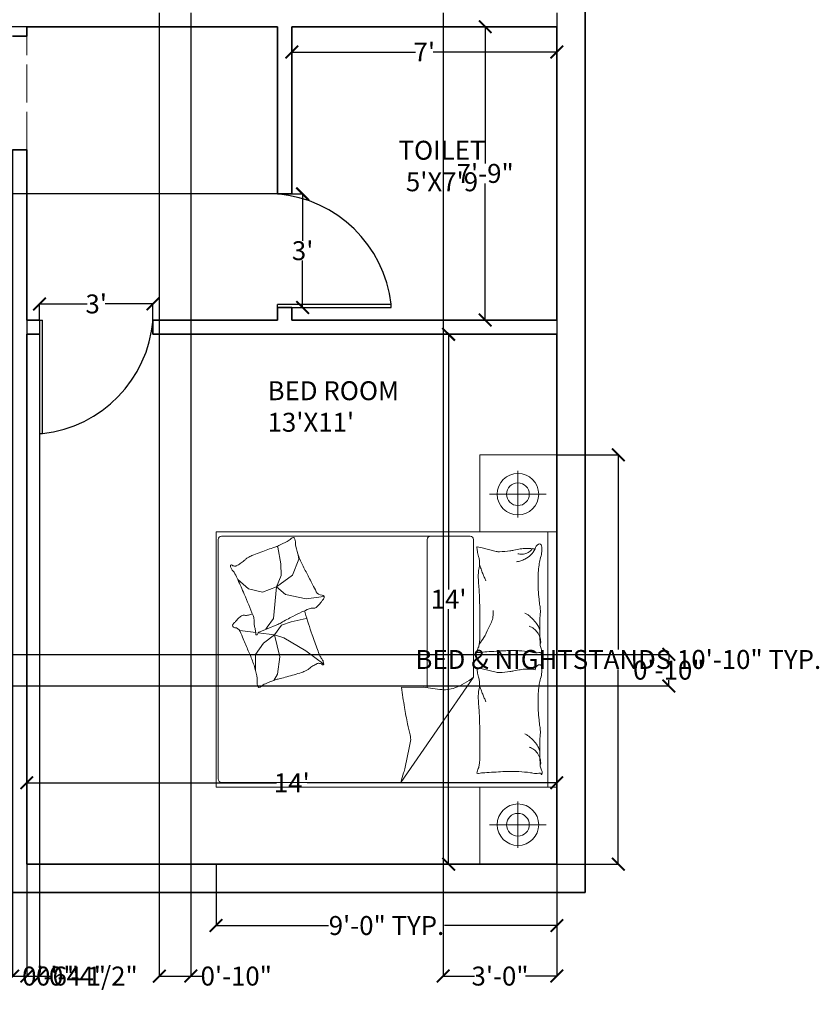
# Model space of a CAD drawing. Units: inches. Extents: x 43 to 543, y 36 to 629.
# Tile 3 of 5: x 290 to 543, y 36 to 348. Entities that reach past the tile are written whole.
import ezdxf

# ---------------------------------------------------------------- set-up
doc = ezdxf.new("R2010")
doc.units = ezdxf.units.IN
doc.header["$MEASUREMENT"] = 0
doc.linetypes.add('ACAD_ISO02W100', pattern=[15, 12, -3])
for name, color, linetype, lineweight in [('A-ANNO-DIMS', 2, 'Continuous', 18), ('A-AREA-IDEN', 7, 'Continuous', 25), ('A-DOOR', 3, 'Continuous', 25), ('A-FURN', 8, 'Continuous', 13), ('A-WALL', 7, 'Continuous', 35), ('A-WALL-OVHD', 7, 'ACAD_ISO02W100', 18)]:
    doc.layers.add(name, color=color, linetype=linetype, lineweight=lineweight)
doc.styles.add('DIM_FONT', font='SIMPLEX.shx', dxfattribs={"width": 0.8})
doc.styles.get("Standard").update_dxf_attribs({"font": 'arial.ttf'})
doc.dimstyles.get("Standard").update_dxf_attribs({"dimtxt": 6, "dimasz": 4, "dimexe": 0.18, "dimexo": 0.0625, "dimgap": 0.09, "dimtad": 0, "dimtih": 1, "dimtoh": 1, "dimdec": 0, "dimzin": 0, "dimdsep": 46, "dimlunit": 4, "dimtxsty": 'Standard', "dimblk": 'ARCHTICK', "dimcen": 0.09, "dimadec": 0, "dimazin": 0, "dimtfac": 1, "dimtdec": 0, "dimtofl": 0, "dimtmove": 0, "dimatfit": 3, "dimldrblk": 'ARCHTICK', "dimfxl": 1, "dimtolj": 1, "dimtzin": 0, "dimarcsym": 1})

# ---------------------------------------------------------------- blocks, each defined once
blk = doc.blocks.new('XDCGFBHJNK')
for p, q in [((549.02, 46.3), (549.02, 41.8)), ((549.02, 46.3), (549.02, 10.3)), ((549.02, 46.3), (550.02, 46.3)), ((550.02, 10.3), (550.02, 46.3)), ((549.02, 10.3), (550.02, 10.3))]:
    blk.add_line(p, q)
blk.add_arc((545.53, 49.68), 39.64, 276.512, 355.1019)
blk = doc.blocks.new('_ArchTick')
at = {"color": 0, "linetype": 'ByBlock', "const_width": 0.15}
blk.add_lwpolyline([(-0.5, -0.5), (0.5, 0.5)], dxfattribs=at)
blk = doc.blocks.new('*D12')
at = {"layer": 'A-ANNO-DIMS', "color": 0, "lineweight": -2, "transparency": 16777216}
for p, q in [((459.82, 248.02), (425.4, 248.02)), ((425.58, 248.02), (425.58, 167.12)), ((425.58, 80.02), (425.58, 160.91)), ((459.82, 80.02), (425.4, 80.02))]:
    blk.add_line(p, q, dxfattribs=at)
at = {"layer": 'Defpoints', "color": 0, "transparency": 16777216}
for p in [(459.88, 248.02), (425.58, 80.02), (459.88, 80.02)]:
    blk.add_point(p, dxfattribs=at)
at = {"layer": 'A-ANNO-DIMS', "color": 0, "lineweight": -2, "transparency": 16777216, "xscale": 4, "yscale": 4, "zscale": 4}
for p, rotation in [((425.58, 248.02), 90), ((425.58, 80.02), 270)]:
    blk.add_blockref('_ArchTick', p, dxfattribs=dict(at, rotation=rotation))
at = {"layer": 'A-ANNO-DIMS', "color": 0, "transparency": 16777216, "insert": (425.58, 164.02), "char_height": 6, "attachment_point": 5}
blk.add_mtext("\\A1;14'", dxfattribs=at)
blk = doc.blocks.new('*D13')
at = {"layer": 'A-ANNO-DIMS', "color": 0, "lineweight": -2, "transparency": 16777216}
for p, q in [((291.88, 80.08), (291.88, 105.97)), ((291.88, 105.79), (370.98, 105.79)), ((459.88, 105.79), (380.78, 105.79)), ((459.88, 80.08), (459.88, 105.97))]:
    blk.add_line(p, q, dxfattribs=at)
at = {"layer": 'Defpoints', "color": 0, "transparency": 16777216}
for p in [(291.88, 105.79), (291.88, 80.02), (459.88, 80.02)]:
    blk.add_point(p, dxfattribs=at)
at = {"layer": 'A-ANNO-DIMS', "color": 0, "lineweight": -2, "transparency": 16777216, "xscale": 4, "yscale": 4, "zscale": 4, "rotation": 180}
blk.add_blockref('_ArchTick', (291.88, 105.79), dxfattribs=at)
at = {"layer": 'A-ANNO-DIMS', "color": 0, "lineweight": -2, "transparency": 16777216, "xscale": 4, "yscale": 4, "zscale": 4}
blk.add_blockref('_ArchTick', (459.88, 105.79), dxfattribs=at)
at = {"layer": 'A-ANNO-DIMS', "color": 0, "transparency": 16777216, "insert": (375.88, 105.79), "char_height": 6, "attachment_point": 5}
blk.add_mtext("\\A1;14'", dxfattribs=at)
blk = doc.blocks.new('*D14')
at = {"layer": 'A-ANNO-DIMS', "color": 0, "lineweight": -2, "transparency": 16777216}
for p, q in [((459.82, 345.52), (437, 345.52)), ((437.18, 345.52), (437.18, 302.17)), ((437.18, 252.52), (437.18, 295.86)), ((459.82, 252.52), (437, 252.52))]:
    blk.add_line(p, q, dxfattribs=at)
at = {"layer": 'Defpoints', "color": 0, "transparency": 16777216}
for p in [(459.88, 345.52), (437.18, 252.52), (459.88, 252.52)]:
    blk.add_point(p, dxfattribs=at)
at = {"layer": 'A-ANNO-DIMS', "color": 0, "lineweight": -2, "transparency": 16777216, "xscale": 4, "yscale": 4, "zscale": 4}
for p, rotation in [((437.18, 345.52), 90), ((437.18, 252.52), 270)]:
    blk.add_blockref('_ArchTick', p, dxfattribs=dict(at, rotation=rotation))
at = {"layer": 'A-ANNO-DIMS', "color": 0, "transparency": 16777216, "insert": (437.18, 299.02), "char_height": 6, "attachment_point": 5}
blk.add_mtext('\\A1;7\'-9"', dxfattribs=at)
blk = doc.blocks.new('*D15')
at = {"layer": 'A-ANNO-DIMS', "color": 0, "lineweight": -2, "transparency": 16777216}
for p, q in [((375.88, 345.45), (375.88, 337.34)), ((459.88, 345.45), (459.88, 337.34)), ((375.88, 337.52), (415.05, 337.52)), ((459.88, 337.52), (420.7, 337.52))]:
    blk.add_line(p, q, dxfattribs=at)
at = {"layer": 'Defpoints', "color": 0, "transparency": 16777216}
for p in [(375.88, 345.52), (459.88, 345.52), (459.88, 337.52)]:
    blk.add_point(p, dxfattribs=at)
at = {"layer": 'A-ANNO-DIMS', "color": 0, "lineweight": -2, "transparency": 16777216, "xscale": 4, "yscale": 4, "zscale": 4, "rotation": 180}
blk.add_blockref('_ArchTick', (375.88, 337.52), dxfattribs=at)
at = {"layer": 'A-ANNO-DIMS', "color": 0, "lineweight": -2, "transparency": 16777216, "xscale": 4, "yscale": 4, "zscale": 4}
blk.add_blockref('_ArchTick', (459.88, 337.52), dxfattribs=at)
at = {"layer": 'A-ANNO-DIMS', "color": 0, "transparency": 16777216, "insert": (417.88, 337.52), "char_height": 6, "attachment_point": 5}
blk.add_mtext("\\A1;7'", dxfattribs=at)
blk = doc.blocks.new('*D20')
at = {"layer": 'A-ANNO-DIMS', "color": 0, "lineweight": -2, "transparency": 16777216}
for p, q in [((295.88, 252.58), (295.88, 257.82)), ((295.88, 257.64), (311.03, 257.64)), ((331.88, 257.64), (316.73, 257.64)), ((331.88, 252.58), (331.88, 257.82))]:
    blk.add_line(p, q, dxfattribs=at)
at = {"layer": 'Defpoints', "color": 0, "transparency": 16777216}
for p in [(295.88, 257.64), (295.88, 252.52), (331.88, 252.52)]:
    blk.add_point(p, dxfattribs=at)
at = {"layer": 'A-ANNO-DIMS', "color": 0, "lineweight": -2, "transparency": 16777216, "xscale": 4, "yscale": 4, "zscale": 4, "rotation": 180}
blk.add_blockref('_ArchTick', (295.88, 257.64), dxfattribs=at)
at = {"layer": 'A-ANNO-DIMS', "color": 0, "lineweight": -2, "transparency": 16777216, "xscale": 4, "yscale": 4, "zscale": 4}
blk.add_blockref('_ArchTick', (331.88, 257.64), dxfattribs=at)
at = {"layer": 'A-ANNO-DIMS', "color": 0, "transparency": 16777216, "insert": (313.88, 257.64), "char_height": 6, "attachment_point": 5}
blk.add_mtext("\\A1;3'", dxfattribs=at)
blk = doc.blocks.new('*D21')
at = {"layer": 'A-ANNO-DIMS', "color": 0, "lineweight": -2, "transparency": 16777216}
for p, q in [((371.44, 292.52), (379.48, 292.52)), ((379.3, 292.52), (379.3, 277.67)), ((379.3, 256.52), (379.3, 271.36)), ((371.44, 256.52), (379.48, 256.52))]:
    blk.add_line(p, q, dxfattribs=at)
at = {"layer": 'Defpoints', "color": 0, "transparency": 16777216}
for p in [(371.38, 292.52), (371.38, 256.52), (379.3, 256.52)]:
    blk.add_point(p, dxfattribs=at)
at = {"layer": 'A-ANNO-DIMS', "color": 0, "lineweight": -2, "transparency": 16777216, "xscale": 4, "yscale": 4, "zscale": 4}
for p, rotation in [((379.3, 292.52), 90), ((379.3, 256.52), 270)]:
    blk.add_blockref('_ArchTick', p, dxfattribs=dict(at, rotation=rotation))
at = {"layer": 'A-ANNO-DIMS', "color": 0, "transparency": 16777216, "insert": (379.3, 274.52), "char_height": 6, "attachment_point": 5}
blk.add_mtext("\\A1;3'", dxfattribs=at)
blk = doc.blocks.new('BED-DOUBLE-WITH-NIGHTSTANDS')
for p, q in [((83.62, 105.4), (83.62, 129.79)), ((83.62, 129.79), (108, 129.79)), ((108, 129.79), (108, 105.4)), ((95.68, 109.93), (95.68, 124.65)), ((104.67, 117.29), (86.69, 117.29)), ((80.54, 104), (1.74, 104)), ((105.17, 105.4), (105.17, 24.4)), ((0.66, 102.92), (0.66, 27.01)), ((19.54, 100.52), (19.19, 100.7)), ((20.47, 95.22), (19.54, 100.52)), ((66.9, 102.92), (66.9, 55.97)), ((81.62, 59.31), (81.62, 102.92)), ((26.22, 96.71), (26.04, 98.01)), ((20.65, 91.51), (20.47, 95.22)), ((24.18, 91.6), (26.22, 96.71)), ((19.17, 87.89), (24.18, 91.6)), ((19.17, 87.89), (20.65, 91.51)), ((10.26, 87.33), (6.88, 90.22)), ((19.17, 87.89), (14.71, 86.21)), ((19.17, 87.89), (18.15, 77.85)), ((21.95, 85.47), (19.17, 87.89)), ((14.71, 86.21), (10.26, 87.33)), ((28.54, 84.08), (21.95, 85.47)), ((34.11, 84.82), (28.54, 84.08)), ((16.2, 75.16), (15.73, 74.51)), ((18.15, 77.85), (16.2, 75.16)), ((18.47, 72.7), (20.71, 75.8)), ((20.71, 75.8), (23.8, 76.86)), ((23.8, 76.86), (28.6, 77.93)), ((12.59, 73.43), (7.48, 74.07)), ((18.47, 72.7), (13.38, 73.34)), ((18.47, 72.7), (15.05, 70.03)), ((21.45, 71.74), (18.47, 72.7)), ((18.47, 72.7), (20.17, 65.76)), ((15.05, 70.03), (12.49, 66.51)), ((28.49, 67.68), (21.45, 71.74)), ((12.49, 66.51), (12.49, 61.49)), ((20.17, 65.76), (19.43, 60.21)), ((34.11, 63.41), (28.49, 67.68)), ((19.43, 60.21), (18.34, 58.27)), ((81.62, 59.31), (58.54, 25.93)), ((1.74, 25.93), (58.54, 25.93)), ((83.62, 24.4), (83.62, 0)), ((108, 0), (108, 24.4)), ((95.68, 19.86), (95.68, 5.14)), ((104.67, 12.5), (86.69, 12.5)), ((83.62, 0), (108, 0))]:
    blk.add_line(p, q)
blk.add_lwpolyline([(0, 105.4), (108, 105.4), (108, 24.4), (0, 24.4)], close=True)
blk.add_lwpolyline([(22.51, 102.26, 0.101392), (23.8, 103.26, -0.223768), (24.5, 103.58, -0.25558), (24.77, 103.43, -0.081563), (25.1, 102.61, -0.071805), (25.18, 101.69, 0.069985), (25.26, 100.74, 0.03546), (26.2, 97.59, 0.029432), (27.82, 93.98, 0.001554), (28.73, 92.24, -0.00152), (29.66, 90.47, -0.004735), (30.6, 88.63, 0.00382), (31.75, 86.35, 0.296001), (33.58, 85.3, -0.649774), (34.16, 84.19, -0.02319), (33.93, 83.92, 0.0288), (33.74, 83.71, 0.005727), (33.46, 83.33, -0.004358), (33.09, 82.83, -0.027528), (32.25, 81.85, -0.046214), (31.67, 81.34, -0.194121), (30.78, 81.12, 0.133719), (29.49, 80.96, 0.011505), (27.21, 79.95, 0.008882), (24.3, 78.53, 0.012426), (20.61, 76.53, -0.033612), (19.21, 75.84), (16.17, 74.6), (13.82, 73.64, 0.224341), (13.11, 72.86, -0.722772), (12.63, 72.85, -0.103513), (12.6, 73.05, 0.053465), (12.59, 73.44, 0.030109), (12.34, 74.68, -0.031436), (12.1, 75.88, -0.05324), (12.08, 76.69, 0.05518), (12.05, 77.48, 0.056271), (11.7, 78.85, 0.0108), (8.92, 85.64, 0.00456), (6.88, 90.22, 0.01125), (5.99, 92.05, 0.069394), (5.31, 93.02, -0.079756), (4.74, 93.88, -0.106399), (4.57, 94.66, -0.328642), (4.73, 94.89, -0.299547), (5.09, 94.79, 0.189917), (5.59, 94.53, 0.033518), (6.15, 94.51, 0.075627), (6.39, 94.55, 0.053489), (6.8, 94.74, 0.017838), (7.94, 95.49, 0.038394), (9.17, 96.51, -0.059529), (10, 97.14, -0.035943), (11.36, 97.82, -0.011245), (15.91, 99.56, -0.006203), (17.99, 100.27, 0.010783), (19.19, 100.7, 0.019485), (19.89, 100.99, 0.005062)], format="xyb", close=True)
for points in [[(101.15, 99.94, -0.263368), (102.17, 101.45, -0.494818), (103.18, 100.96, -0.049225), (103.27, 100, -0.036831), (103.18, 98.73, -0.031893), (102.74, 96.68, 0.035782), (102.36, 94.84, 0.032941), (102.04, 90, 0.026564), (102.36, 84, 0.017905), (102.65, 81.97, -0.033397), (102.77, 80.88, -0.03204), (102.73, 78.88, 0.018442), (102.57, 75.4, 0.010837), (102.61, 71.91, 0.014624), (102.77, 69.32, 0.111249), (103.17, 68.1, -0.153708), (103.38, 67.19, -0.076444), (103.29, 66.79, -0.215512), (103.18, 66.68, -0.585858), (103.02, 66.83, 0.363489), (102.88, 67.09, 0.191716), (102.25, 67.09, -0.129675), (101.36, 66.99, -0.01735), (100.45, 67.15, 0.019326), (99.63, 67.29, 0.018818), (95.94, 67.65, 0.021828), (92.74, 67.7, 0.006204), (90.91, 67.62, 0.001963), (85.14, 67.29, 0.028341), (83.19, 67.06, -0.117014), (82.71, 67.09, -0.36606), (82.66, 67.17, -0.03973), (82.81, 67.9, -0.048309), (83.11, 68.64, 0.062981), (83.32, 69.22, 0.04058), (83.5, 70.48, 0.014345), (83.62, 74.08, 0.005484), (83.58, 80.86, 0.007153), (83.42, 86.05, 0.008762), (83.27, 88.35, -0.008153), (83.12, 90.82, -0.06251), (83.35, 93.9, 0.078669), (83.46, 96.36, 0.047825), (83.21, 97.57, -0.034494), (82.81, 99.23, -0.023571), (82.65, 100.6, -0.510228), (82.71, 100.65), (84.33, 100.25), (88.79, 99.13, 0.073041), (89.85, 99.03, 0.023305), (93.15, 99.33, 0.018299), (94.38, 99.55, -0.01097), (96.43, 99.95, -0.042281), (98.29, 100.11, -0.027201), (101.17, 99.95)], [(101.15, 99.95, -0.077379), (99.79, 98.07, -0.077379), (97.91, 96.7, -0.047525), (96.58, 96.16, -0.047525), (95.17, 95.89)], [(100.29, 100.03, -0.05369), (99.59, 99.27, -0.070312), (98.92, 98.83, -0.015448), (98.46, 98.63, -0.013244), (97.91, 98.42, -0.082127), (96.93, 98.26, -0.064164), (95.68, 98.42)], [(83.5, 95.06, 0.009729), (83.99, 93.59, 0.009729), (84.53, 92.13, 0.007971), (85.02, 90.96, 0.007971), (85.55, 89.8)], [(28.06, 80.34, 0.025626), (28.21, 79.72, 0.0108), (30.46, 72.73, 0.00456), (32.14, 68.01, 0.01125), (32.88, 66.11, 0.069394), (33.49, 65.1, -0.079756), (33.99, 64.2, -0.106399), (34.11, 63.41, -0.328642), (33.92, 63.19, -0.299547), (33.57, 63.32, 0.189917), (33.1, 63.62, 0.033518), (32.54, 63.68, 0.075627), (32.29, 63.65, 0.053489), (31.87, 63.49, 0.017838), (30.68, 62.84, 0.038394), (29.37, 61.91, -0.059529), (28.5, 61.35, -0.035943), (27.09, 60.78, -0.011245), (22.42, 59.39, -0.006203), (20.29, 58.84, 0.010783), (19.06, 58.51, 0.019485), (18.34, 58.27, 0.005062), (15.63, 57.21, 0.101392), (14.27, 56.3, -0.223768), (13.54, 56.04, -0.25558), (13.29, 56.21, -0.081563), (13.02, 57.06, -0.071805), (13.01, 57.98, 0.069985), (13.01, 58.93, 0.03546), (12.31, 62.14, 0.029432), (10.97, 65.87, 0.001554), (10.2, 67.67, -0.00152), (9.41, 69.51, -0.004735), (8.61, 71.41, 0.00382), (7.64, 73.78, 0.296001), (5.89, 74.96, -0.649774), (5.41, 76.12, -0.02319), (5.66, 76.36, 0.0288), (5.85, 76.56, 0.005727), (6.17, 76.91, -0.004358), (6.58, 77.38, -0.027528), (7.49, 78.3, -0.046214), (8.1, 78.76, -0.194121), (9, 78.91, 0.133719), (10.3, 78.98, 0.005779), (11.49, 79.38, 0.008882)], [(83.42, 69.72, 0.016108), (84.84, 71.83, 0.024599), (85.65, 73.27, 0.009477), (86.91, 75.92, 0.015937), (87.57, 77.53, 0.072521), (87.77, 78.41, 0.033339), (87.78, 80.37)], [(102.57, 74.35, 0.027842), (101.99, 75.64, 0.048685), (101.56, 76.32, 0.023666), (100.24, 77.82, 0.031223), (99.13, 78.85, 0.046801), (98.71, 79.13, 0.023191), (97.81, 79.56)], [(102.88, 69.93, 0.088153), (102.68, 71.79, 0.088153), (101.86, 73.48, 0.077547), (100.7, 74.65, 0.077547), (99.23, 75.4)], [(101.15, 61.64, -0.263368), (102.17, 63.15, -0.494818), (103.18, 62.66, -0.049225), (103.27, 61.7, -0.036831), (103.18, 60.43, -0.031893), (102.74, 58.38, 0.035782), (102.36, 56.55, 0.032941), (102.04, 51.7, 0.026564), (102.36, 45.7, 0.017905), (102.65, 43.67, -0.033397), (102.77, 42.58, -0.03204), (102.73, 40.58, 0.018442), (102.57, 37.1, 0.010837), (102.61, 33.61, 0.014624), (102.77, 31.02, 0.111249), (103.17, 29.8, -0.153708), (103.38, 28.89, -0.076444), (103.29, 28.49, -0.215512), (103.18, 28.38, -0.585858), (103.02, 28.53, 0.363489), (102.88, 28.79, 0.191716), (102.25, 28.79, -0.129675), (101.36, 28.69, -0.01735), (100.45, 28.85, 0.019326), (99.63, 28.99, 0.018818), (95.94, 29.35, 0.021828), (92.74, 29.4, 0.006204), (90.91, 29.32, 0.001963), (85.14, 28.99, 0.028341), (83.19, 28.76, -0.117014), (82.71, 28.79, -0.36606), (82.66, 28.87, -0.03973), (82.81, 29.6, -0.048309), (83.11, 30.34, 0.062981), (83.32, 30.92, 0.04058), (83.5, 32.18, 0.014345), (83.62, 35.79, 0.005484), (83.58, 42.56, 0.007153), (83.42, 47.75, 0.008762), (83.27, 50.05, -0.008153), (83.12, 52.52, -0.06251), (83.35, 55.6, 0.078669), (83.46, 58.06, 0.047825), (83.21, 59.27, -0.034494), (82.81, 60.93, -0.023571), (82.65, 62.3, -0.510228), (82.71, 62.35), (84.33, 61.95), (88.79, 60.83, 0.073041), (89.85, 60.73, 0.023305), (93.15, 61.04, 0.018299), (94.38, 61.26, -0.01097), (96.43, 61.65, -0.042281), (98.29, 61.81, -0.027201), (101.17, 61.65)], [(81.62, 59.31, -0.085272), (75.67, 55.89, -0.124044), (70.95, 55.39), (65.79, 56.13), (58.77, 56.03)], [(83.5, 56.76, 0.009729), (83.99, 55.29, 0.009729), (84.53, 53.84, 0.007971), (85.02, 52.66, 0.007971), (85.55, 51.5)], [(58.77, 56.03, 0.007867), (59.73, 49.68, 0.009508), (60.7, 44.46, 0.006616), (61.48, 40.95, -0.023828), (61.66, 39.97, -0.080713), (61.63, 38.96, -0.009591), (59.91, 30.72, -0.013133), (59.44, 28.91, -0.007859), (58.54, 25.93)], [(102.57, 36.06, 0.027842), (101.99, 37.34, 0.048685), (101.56, 38.02, 0.023666), (100.24, 39.52, 0.031223), (99.13, 40.55, 0.046801), (98.71, 40.83, 0.023191), (97.81, 41.26)], [(102.88, 31.63, 0.088153), (102.68, 33.49, 0.088153), (101.86, 35.18, 0.077547), (100.7, 36.35, 0.077547), (99.23, 37.1)]]:
    blk.add_lwpolyline(points, format="xyb")
for centre, radius in [((95.68, 117.29), 6.58), ((95.68, 117.29), 3.6), ((95.68, 12.5), 6.58), ((95.68, 12.5), 3.6)]:
    blk.add_circle(centre, radius)
for centre, start, end in [((1.74, 102.92), 90, 180), ((67.98, 102.92), 90, 180), ((80.54, 102.92), 0, 90), ((1.74, 27.01), 180, 270)]:
    blk.add_arc(centre, 1.08, start, end)
at = {"style": 'DIM_FONT', "width": 0.8, "flags": 9}
for tag in ['YSIZE', 'XSIZE']:
    blk.add_attdef(tag, (108, 105.4), '', height=0.027, rotation=270, dxfattribs=at)
blk = doc.blocks.new('*D27')
at = {"layer": 'A-ANNO-DIMS', "color": 0, "lineweight": -2, "transparency": 16777216}
for p, q in [((459.97, 209.81), (479.55, 209.81)), ((479.37, 209.81), (479.37, 148.12)), ((479.37, 80.02), (479.37, 141.7)), ((459.97, 80.02), (479.55, 80.02))]:
    blk.add_line(p, q, dxfattribs=at)
at = {"layer": 'Defpoints', "color": 0, "transparency": 16777216}
for p in [(459.9, 209.81), (479.37, 209.81), (459.9, 80.02)]:
    blk.add_point(p, dxfattribs=at)
at = {"layer": 'A-ANNO-DIMS', "color": 0, "lineweight": -2, "transparency": 16777216, "xscale": 4, "yscale": 4, "zscale": 4}
for p, rotation in [((479.37, 209.81), 90), ((479.37, 80.02), 270)]:
    blk.add_blockref('_ArchTick', p, dxfattribs=dict(at, rotation=rotation))
at = {"layer": 'A-ANNO-DIMS', "color": 0, "transparency": 16777216, "insert": (479.37, 144.91), "char_height": 6, "attachment_point": 5}
blk.add_mtext('\\A1;BED & NIGHTSTANDS 10\'-10" TYP.', dxfattribs=at)
blk = doc.blocks.new('*D28')
at = {"layer": 'A-ANNO-DIMS', "color": 0, "lineweight": -2, "transparency": 16777216}
for p, q in [((351.88, 79.95), (351.88, 60.37)), ((459.9, 79.95), (459.9, 60.37)), ((351.88, 60.55), (387.51, 60.55)), ((459.9, 60.55), (424.27, 60.55))]:
    blk.add_line(p, q, dxfattribs=at)
at = {"layer": 'Defpoints', "color": 0, "transparency": 16777216}
for p in [(351.88, 80.02), (459.9, 80.02), (459.9, 60.55)]:
    blk.add_point(p, dxfattribs=at)
at = {"layer": 'A-ANNO-DIMS', "color": 0, "lineweight": -2, "transparency": 16777216, "xscale": 4, "yscale": 4, "zscale": 4, "rotation": 180}
blk.add_blockref('_ArchTick', (351.88, 60.55), dxfattribs=at)
at = {"layer": 'A-ANNO-DIMS', "color": 0, "lineweight": -2, "transparency": 16777216, "xscale": 4, "yscale": 4, "zscale": 4}
blk.add_blockref('_ArchTick', (459.9, 60.55), dxfattribs=at)
at = {"layer": 'A-ANNO-DIMS', "color": 0, "transparency": 16777216, "insert": (405.89, 60.55), "char_height": 6, "attachment_point": 5}
blk.add_mtext('\\A1;9\'-0" TYP.', dxfattribs=at)
blk = doc.blocks.new('*D36')
at = {"layer": 'A-ANNO-DIMS', "color": 0, "lineweight": -2, "transparency": 16777216}
for p, q in [((459.88, 363.72), (459.88, 356.4)), ((468.88, 363.72), (468.88, 356.4)), ((459.88, 356.58), (468.88, 356.58)), ((468.88, 356.58), (472.88, 356.58))]:
    blk.add_line(p, q, dxfattribs=at)
at = {"layer": 'Defpoints', "color": 0, "transparency": 16777216}
for p in [(459.88, 363.78), (468.88, 363.78), (468.88, 356.58)]:
    blk.add_point(p, dxfattribs=at)
at = {"layer": 'A-ANNO-DIMS', "color": 0, "lineweight": -2, "transparency": 16777216, "xscale": 4, "yscale": 4, "zscale": 4, "rotation": 180}
blk.add_blockref('_ArchTick', (459.88, 356.58), dxfattribs=at)
at = {"layer": 'A-ANNO-DIMS', "color": 0, "lineweight": -2, "transparency": 16777216, "xscale": 4, "yscale": 4, "zscale": 4}
blk.add_blockref('_ArchTick', (468.88, 356.58), dxfattribs=at)
at = {"layer": 'A-ANNO-DIMS', "color": 0, "transparency": 16777216, "insert": (491.25, 356.58), "char_height": 6, "attachment_point": 5}
blk.add_mtext('\\A1;0\'-9" TYP.', dxfattribs=at)
blk = doc.blocks.new('*D42')
at = {"layer": 'A-ANNO-DIMS', "color": 0, "lineweight": -2, "transparency": 16777216}
for p, q in [((281.38, 156.45), (281.38, 44.34)), ((287.38, 156.45), (287.38, 44.34)), ((281.38, 44.52), (287.38, 44.52)), ((287.38, 44.52), (291.38, 44.52))]:
    blk.add_line(p, q, dxfattribs=at)
at = {"layer": 'Defpoints', "color": 0, "transparency": 16777216}
for p in [(281.38, 156.52), (287.38, 156.52), (287.38, 44.52)]:
    blk.add_point(p, dxfattribs=at)
at = {"layer": 'A-ANNO-DIMS', "color": 0, "lineweight": -2, "transparency": 16777216, "xscale": 4, "yscale": 4, "zscale": 4, "rotation": 180}
blk.add_blockref('_ArchTick', (281.38, 44.52), dxfattribs=at)
at = {"layer": 'A-ANNO-DIMS', "color": 0, "lineweight": -2, "transparency": 16777216, "xscale": 4, "yscale": 4, "zscale": 4}
blk.add_blockref('_ArchTick', (287.38, 44.52), dxfattribs=at)
at = {"layer": 'A-ANNO-DIMS', "color": 0, "transparency": 16777216, "insert": (299.44, 44.52), "char_height": 6, "attachment_point": 5}
blk.add_mtext('\\A1;0\'-6"', dxfattribs=at)
blk = doc.blocks.new('*D47')
at = {"layer": 'A-ANNO-DIMS', "color": 0, "lineweight": -2, "transparency": 16777216}
for p, q in [((423.88, 349.95), (423.88, 44.34)), ((459.88, 349.95), (459.88, 44.34)), ((423.88, 44.52), (433.81, 44.52)), ((459.88, 44.52), (449.94, 44.52))]:
    blk.add_line(p, q, dxfattribs=at)
at = {"layer": 'Defpoints', "color": 0, "transparency": 16777216}
for p in [(423.88, 350.02), (459.88, 350.02), (459.88, 44.52)]:
    blk.add_point(p, dxfattribs=at)
at = {"layer": 'A-ANNO-DIMS', "color": 0, "lineweight": -2, "transparency": 16777216, "xscale": 4, "yscale": 4, "zscale": 4, "rotation": 180}
blk.add_blockref('_ArchTick', (423.88, 44.52), dxfattribs=at)
at = {"layer": 'A-ANNO-DIMS', "color": 0, "lineweight": -2, "transparency": 16777216, "xscale": 4, "yscale": 4, "zscale": 4}
blk.add_blockref('_ArchTick', (459.88, 44.52), dxfattribs=at)
at = {"layer": 'A-ANNO-DIMS', "color": 0, "transparency": 16777216, "insert": (441.88, 44.52), "char_height": 6, "attachment_point": 5}
blk.add_mtext('\\A1;3\'-0"', dxfattribs=at)
blk = doc.blocks.new('*D48')
at = {"layer": 'A-ANNO-DIMS', "color": 0, "lineweight": -2, "transparency": 16777216}
for p, q in [((333.88, 349.95), (333.88, 44.34)), ((343.88, 349.95), (343.88, 44.34)), ((333.88, 44.52), (343.88, 44.52)), ((343.88, 44.52), (347.88, 44.52))]:
    blk.add_line(p, q, dxfattribs=at)
at = {"layer": 'Defpoints', "color": 0, "transparency": 16777216}
for p in [(333.88, 350.02), (343.88, 350.02), (343.88, 44.52)]:
    blk.add_point(p, dxfattribs=at)
at = {"layer": 'A-ANNO-DIMS', "color": 0, "lineweight": -2, "transparency": 16777216, "xscale": 4, "yscale": 4, "zscale": 4, "rotation": 180}
blk.add_blockref('_ArchTick', (333.88, 44.52), dxfattribs=at)
at = {"layer": 'A-ANNO-DIMS', "color": 0, "lineweight": -2, "transparency": 16777216, "xscale": 4, "yscale": 4, "zscale": 4}
blk.add_blockref('_ArchTick', (343.88, 44.52), dxfattribs=at)
at = {"layer": 'A-ANNO-DIMS', "color": 0, "transparency": 16777216, "insert": (358.27, 44.52), "char_height": 6, "attachment_point": 5}
blk.add_mtext('\\A1;0\'-10"', dxfattribs=at)
blk = doc.blocks.new('*D49')
at = {"layer": 'A-ANNO-DIMS', "color": 0, "lineweight": -2, "transparency": 16777216}
for p, q in [((371.32, 345.52), (58.2, 345.52)), ((58.38, 345.52), (58.38, 322.16)), ((58.38, 292.52), (58.38, 315.88)), ((371.32, 292.52), (58.2, 292.52))]:
    blk.add_line(p, q, dxfattribs=at)
at = {"layer": 'Defpoints', "color": 0, "transparency": 16777216}
for p in [(58.38, 345.52), (371.38, 345.52), (371.38, 292.52)]:
    blk.add_point(p, dxfattribs=at)
at = {"layer": 'A-ANNO-DIMS', "color": 0, "lineweight": -2, "transparency": 16777216, "xscale": 4, "yscale": 4, "zscale": 4}
for p, rotation in [((58.38, 345.52), 90), ((58.38, 292.52), 270)]:
    blk.add_blockref('_ArchTick', p, dxfattribs=dict(at, rotation=rotation))
at = {"layer": 'A-ANNO-DIMS', "color": 0, "transparency": 16777216, "insert": (58.38, 319.02), "char_height": 6, "attachment_point": 5}
blk.add_mtext('\\A1;4\'-5"', dxfattribs=at)
blk = doc.blocks.new('*D62')
at = {"layer": 'A-ANNO-DIMS', "color": 0, "lineweight": -2, "transparency": 16777216}
for p, q in [((291.88, 252.45), (291.88, 44.34)), ((295.88, 252.45), (295.88, 44.34)), ((291.88, 44.52), (295.88, 44.52)), ((295.88, 44.52), (299.88, 44.52))]:
    blk.add_line(p, q, dxfattribs=at)
at = {"layer": 'Defpoints', "color": 0, "transparency": 16777216}
for p in [(291.88, 252.52), (295.88, 252.52), (295.88, 44.52)]:
    blk.add_point(p, dxfattribs=at)
at = {"layer": 'A-ANNO-DIMS', "color": 0, "lineweight": -2, "transparency": 16777216, "xscale": 4, "yscale": 4, "zscale": 4, "rotation": 180}
blk.add_blockref('_ArchTick', (291.88, 44.52), dxfattribs=at)
at = {"layer": 'A-ANNO-DIMS', "color": 0, "lineweight": -2, "transparency": 16777216, "xscale": 4, "yscale": 4, "zscale": 4}
blk.add_blockref('_ArchTick', (295.88, 44.52), dxfattribs=at)
at = {"layer": 'A-ANNO-DIMS', "color": 0, "transparency": 16777216, "insert": (307.94, 44.52), "char_height": 6, "attachment_point": 5}
blk.add_mtext('\\A1;0\'-4"', dxfattribs=at)
blk = doc.blocks.new('*D66')
at = {"layer": 'A-ANNO-DIMS', "color": 0, "lineweight": -2, "transparency": 16777216}
for p, q in [((287.44, 146.52), (495.56, 146.52)), ((495.38, 146.52), (495.38, 144.67)), ((495.38, 136.52), (495.38, 138.36)), ((287.44, 136.52), (495.56, 136.52))]:
    blk.add_line(p, q, dxfattribs=at)
at = {"layer": 'Defpoints', "color": 0, "transparency": 16777216}
for p in [(287.38, 146.52), (495.38, 146.52), (287.38, 136.52)]:
    blk.add_point(p, dxfattribs=at)
at = {"layer": 'A-ANNO-DIMS', "color": 0, "lineweight": -2, "transparency": 16777216, "xscale": 4, "yscale": 4, "zscale": 4}
for p, rotation in [((495.38, 146.52), 90), ((495.38, 136.52), 270)]:
    blk.add_blockref('_ArchTick', p, dxfattribs=dict(at, rotation=rotation))
at = {"layer": 'A-ANNO-DIMS', "color": 0, "transparency": 16777216, "insert": (495.38, 141.52), "char_height": 6, "attachment_point": 5}
blk.add_mtext('\\A1;0\'-10"', dxfattribs=at)
blk = doc.blocks.new('*D67')
at = {"layer": 'A-ANNO-DIMS', "color": 0, "lineweight": -2, "transparency": 16777216}
for p, q in [((287.38, 306.45), (287.38, 44.34)), ((291.88, 306.45), (291.88, 44.34)), ((287.38, 44.52), (291.88, 44.52)), ((291.88, 44.52), (295.88, 44.52))]:
    blk.add_line(p, q, dxfattribs=at)
at = {"layer": 'Defpoints', "color": 0, "transparency": 16777216}
for p in [(287.38, 306.52), (291.88, 306.52), (291.88, 44.52)]:
    blk.add_point(p, dxfattribs=at)
at = {"layer": 'A-ANNO-DIMS', "color": 0, "lineweight": -2, "transparency": 16777216, "xscale": 4, "yscale": 4, "zscale": 4, "rotation": 180}
blk.add_blockref('_ArchTick', (287.38, 44.52), dxfattribs=at)
at = {"layer": 'A-ANNO-DIMS', "color": 0, "lineweight": -2, "transparency": 16777216, "xscale": 4, "yscale": 4, "zscale": 4}
blk.add_blockref('_ArchTick', (291.88, 44.52), dxfattribs=at)
at = {"layer": 'A-ANNO-DIMS', "color": 0, "transparency": 16777216, "insert": (310.93, 44.52), "char_height": 6, "attachment_point": 5}
blk.add_mtext('\\A1;0\'-4 1/2"', dxfattribs=at)

msp = doc.modelspace()

# ---------------------------------------------------------------- linework, layer by layer
at = {"layer": 'A-WALL'}
for p, q in [((468.88, 599.02), (468.88, 71.02)), ((291.88, 345.52), (291.88, 342.52)), ((291.88, 345.52), (371.38, 345.52)), ((371.38, 345.52), (371.38, 306.52)), ((375.88, 345.52), (375.88, 306.52)), ((375.88, 345.52), (459.88, 345.52)), ((459.88, 345.52), (459.88, 252.52)), ((287.38, 342.52), (291.88, 342.52)), ((287.38, 306.52), (291.88, 306.52)), ((291.88, 306.52), (291.88, 252.52)), ((371.38, 306.52), (371.38, 292.52)), ((375.88, 306.52), (375.88, 292.52)), ((375.88, 292.52), (371.38, 292.52)), ((375.88, 256.52), (371.38, 256.52)), ((371.38, 256.52), (371.38, 252.52)), ((375.88, 256.52), (375.88, 252.52)), ((295.88, 252.52), (291.88, 252.52)), ((371.38, 252.52), (331.88, 252.52)), ((331.88, 252.52), (331.88, 248.02)), ((459.88, 252.52), (375.88, 252.52)), ((291.88, 248.02), (291.88, 80.02)), ((295.88, 248.02), (291.88, 248.02)), ((459.88, 248.02), (331.88, 248.02)), ((459.88, 248.02), (459.88, 80.02)), ((459.88, 80.02), (291.88, 80.02)), ((468.88, 71.02), (84.88, 71.02))]:
    msp.add_line(p, q, dxfattribs=at)
at = {"layer": 'A-WALL-OVHD'}
for p, q in [((291.88, 342.52), (287.38, 342.52)), ((291.88, 306.52), (291.88, 342.52))]:
    msp.add_line(p, q, dxfattribs=at)

# ---------------------------------------------------------------- block references
at = {"layer": 'A-DOOR', "rotation": 90}
msp.add_blockref('XDCGFBHJNK', (417.67, -292.51), dxfattribs=at)
at = {"layer": 'A-DOOR'}
msp.add_blockref('XDCGFBHJNK', (-253.14, 206.22), dxfattribs=at)
at = {"layer": 'A-FURN'}
msp.add_blockref('BED-DOUBLE-WITH-NIGHTSTANDS', (351.88, 80.02), dxfattribs=at)

# ---------------------------------------------------------------- texts
at = {"layer": 'A-AREA-IDEN', "char_height": 6, "attachment_point": 1}
for s, width, insert in [("\\pxqc;TOILET\\P5'X7'9", 52.429, (397.26, 309.37)), ("BED ROOM\\P13'X11' ", 90.4757, (368.21, 233.12))]:
    msp.add_mtext_dynamic_manual_height_columns(s, width=width, gutter_width=30, heights=[0], dxfattribs=dict(at, insert=insert))

# ---------------------------------------------------------------- dimensions: what is measured, and where the dimension line sits
at = {"layer": 'A-ANNO-DIMS'}
for base, p1, p2, picture, middle in [((468.88, 356.58), (459.88, 363.78), (468.88, 363.78), '*D36', (491.25, 356.58)), ((459.9, 60.55), (351.88, 80.02), (459.9, 80.02), '*D28', (405.89, 60.55))]:
    dim = msp.add_linear_dim(base=base, p1=p1, p2=p2, text='<> TYP.', dimstyle='Standard', override={"dimdec": 1, "dimlfac": 1, "dimrnd": 0, "dimzin": 1, "dimdsep": 46, "dimlunit": 4, "dimfrac": 2}, dxfattribs=at)
    dim.commit()
    dim.dimension.update_dxf_attribs({"geometry": picture, "text_midpoint": middle})
for base, p1, p2, override, picture, middle in [((343.88, 44.52), (333.88, 350.02), (343.88, 350.02), {"dimdec": 1, "dimlfac": 1, "dimrnd": 0, "dimzin": 1, "dimdsep": 46, "dimlunit": 4, "dimfrac": 2}, '*D48', (358.27, 44.52)), ((459.88, 44.52), (423.88, 350.02), (459.88, 350.02), {"dimdec": 1, "dimlfac": 1, "dimrnd": 0, "dimzin": 1, "dimdsep": 46, "dimlunit": 4, "dimfrac": 2}, '*D47', (441.88, 44.52)), ((459.88, 337.52), (375.88, 345.52), (459.88, 345.52), {"dimclrd": 0, "dimclre": 0, "dimclrt": 0}, '*D15', (417.88, 337.52)), ((291.88, 44.52), (287.38, 306.52), (291.88, 306.52), {"dimdec": 1, "dimlfac": 1, "dimrnd": 0, "dimzin": 1, "dimdsep": 46, "dimlunit": 4, "dimfrac": 2}, '*D67', (310.93, 44.52)), ((295.88, 257.64), (331.88, 252.52), (295.88, 252.52), {"dimclrd": 0, "dimclre": 0, "dimclrt": 0}, '*D20', (313.88, 257.64)), ((295.88, 44.52), (291.88, 252.52), (295.88, 252.52), {"dimdec": 1, "dimlfac": 1, "dimrnd": 0, "dimzin": 1, "dimdsep": 46, "dimlunit": 4, "dimfrac": 2}, '*D62', (307.94, 44.52)), ((287.38, 44.52), (281.38, 156.52), (287.38, 156.52), {"dimdec": 1, "dimlfac": 1, "dimrnd": 0, "dimzin": 1, "dimdsep": 46, "dimlunit": 4, "dimfrac": 2}, '*D42', (299.44, 44.52)), ((291.88, 105.79), (459.88, 80.02), (291.88, 80.02), {"dimclrd": 0, "dimclre": 0, "dimclrt": 0}, '*D13', (375.88, 105.79))]:
    dim = msp.add_linear_dim(base=base, p1=p1, p2=p2, dimstyle='Standard', override=override, dxfattribs=at)
    dim.commit()
    dim.dimension.update_dxf_attribs({"geometry": picture, "text_midpoint": middle})
for base, p1, p2, override, picture, middle in [((58.38, 345.52), (371.38, 292.52), (371.38, 345.52), {"dimdec": 1, "dimlfac": 1, "dimrnd": 0, "dimzin": 1, "dimdsep": 46, "dimlunit": 4, "dimfrac": 2}, '*D49', (58.38, 319.02)), ((437.18, 252.52), (459.88, 345.52), (459.88, 252.52), {"dimclrd": 0, "dimclre": 0, "dimclrt": 0}, '*D14', (437.18, 299.02)), ((379.3, 256.52), (371.38, 292.52), (371.38, 256.52), {"dimclrd": 0, "dimclre": 0, "dimclrt": 0}, '*D21', (379.3, 274.52)), ((425.58, 80.02), (459.88, 248.02), (459.88, 80.02), {"dimclrd": 0, "dimclre": 0, "dimclrt": 0}, '*D12', (425.58, 164.02)), ((495.38, 146.52), (287.38, 136.52), (287.38, 146.52), {"dimdec": 1, "dimlfac": 1, "dimrnd": 0, "dimzin": 1, "dimdsep": 46, "dimlunit": 4, "dimfrac": 2}, '*D66', (495.38, 141.52))]:
    dim = msp.add_linear_dim(base=base, p1=p1, p2=p2, angle=90, dimstyle='Standard', override=override, dxfattribs=at)
    dim.commit()
    dim.dimension.update_dxf_attribs({"geometry": picture, "text_midpoint": middle})
dim = msp.add_linear_dim(base=(479.37, 209.81), p1=(459.9, 80.02), p2=(459.9, 209.81), angle=90, text='BED & NIGHTSTANDS <> TYP.', dimstyle='Standard', override={"dimdec": 1, "dimlfac": 1, "dimrnd": 0, "dimzin": 1, "dimdsep": 46, "dimlunit": 4, "dimfrac": 2}, dxfattribs=at)
dim.commit()
dim.dimension.update_dxf_attribs({"geometry": '*D27', "text_midpoint": (479.37, 144.91)})

doc.saveas('drawing.dxf')
